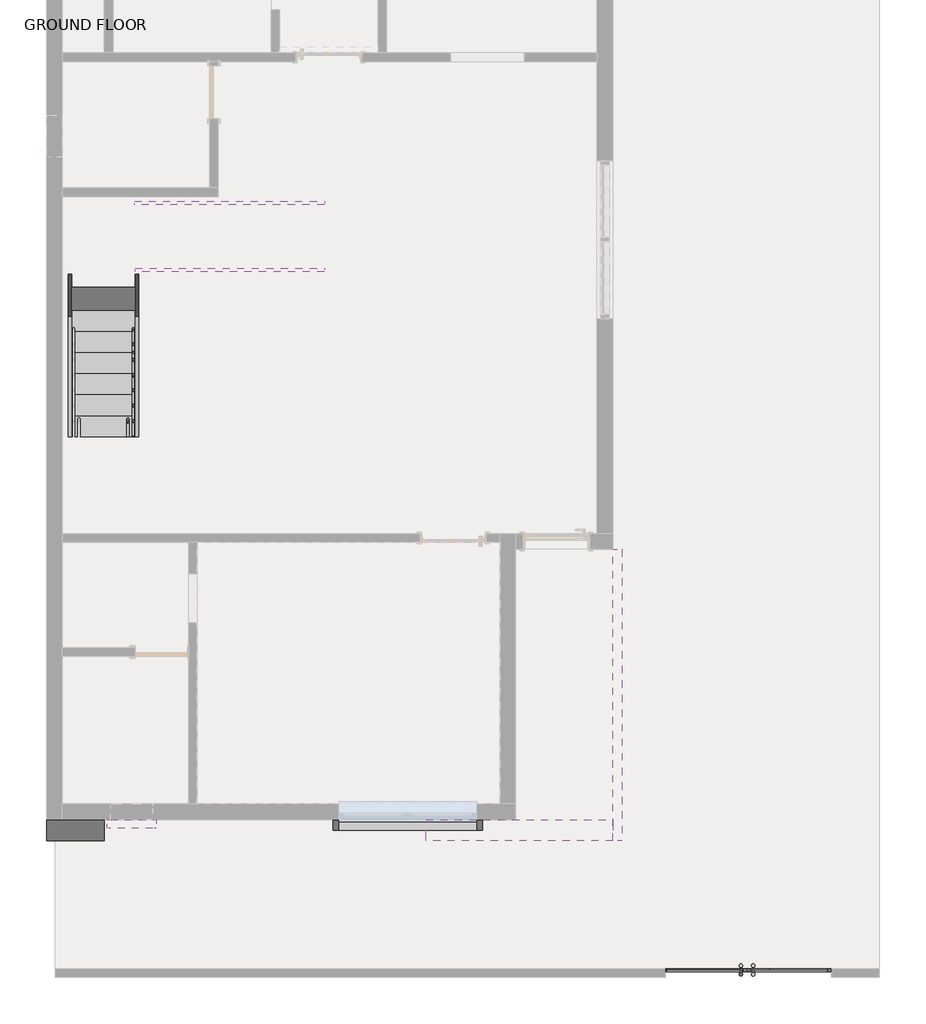
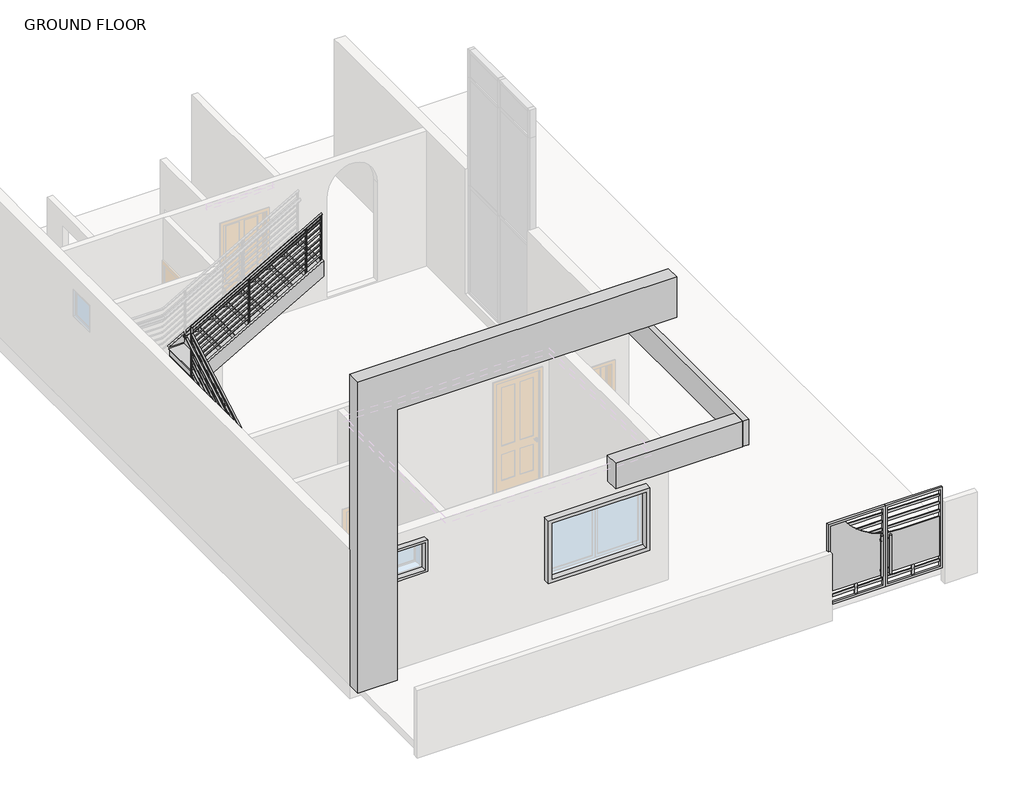
# One storey, part 3 of 3: 6 proxies, 4 members, 1 railing, 1 stair flight.
"""IFC4 building model written with IfcOpenShell, lengths in millimetres."""

from ifc_helpers import new_model, si_unit, frame, origin, place, context, project, spatial, polyline, circle_curve, ellipse_curve, outline, extrude, transform, mapped, element, save
from ifc_brep_helpers import plane_surface, cylinder_surface, advanced_brep
from components import generic_models_113f6068, generic_models_1_generic_models_1_e6ddf01a, generic_models_4_generic_models_3_1a75a499, generic_models_6_generic_models_6_7c639092, generic_models_8_generic_models_8_1b8929a2, wall_frame_wall_frame_a6ba02d1, stair_flight_5496a8fe

model = new_model("IFC4")

# Units and contexts
model_context = context("Model", 3, world=origin())
ifc_project = project(units=[si_unit("LENGTHUNIT", "METRE", prefix="MILLI")], contexts=[model_context])

# Site, building, storey
site = spatial("IfcSite", under=ifc_project)
building = spatial("IfcBuilding", under=site)
storey = spatial("IfcBuildingStorey", under=building, Name="GROUND FLOOR", Elevation=304.8)

# Proxies
placement = place(None, origin())
generic_models_shape = generic_models_113f6068(model_context)
element("IfcBuildingElementProxy", 1, Name="Generic Models", at=placement, inside=storey, context=model_context, shape_type="MappedRepresentation", body=[
    mapped(generic_models_shape, transform((2838.426752, -5931.4866303, 304.8), x_axis=(1.0, 0.0, 0.0), y_axis=(0.0, 1.0, 0.0), z_axis=(0.0, 0.0, 1.0))),
])
generic_models_1_generic_models_1_shape = generic_models_1_generic_models_1_e6ddf01a(model_context)
element("IfcBuildingElementProxy", 2, Name="Generic Models 2 : Generic Models 1", ObjectType="Generic Models 2 : Generic Models 1", at=placement, inside=storey, context=model_context, shape_type="MappedRepresentation", body=[
    mapped(generic_models_1_generic_models_1_shape, transform((0.0, 0.0, -3048.0), x_axis=(1.0, 0.0, 0.0), y_axis=(0.0, 1.0, 0.0), z_axis=(0.0, 0.0, 1.0))),
])
generic_models_4_generic_models_3_shape = generic_models_4_generic_models_3_1a75a499(model_context)
element("IfcBuildingElementProxy", 3, Name="Generic Models 4 : Generic Models 3", ObjectType="Generic Models 4 : Generic Models 3", at=placement, inside=storey, context=model_context, shape_type="MappedRepresentation", body=[
    mapped(generic_models_4_generic_models_3_shape, transform((0.0, 0.0, 0.0), x_axis=(1.0, 0.0, 0.0), y_axis=(0.0, 1.0, 0.0), z_axis=(0.0, 0.0, 1.0))),
])
generic_models_6_generic_models_6_shape = generic_models_6_generic_models_6_7c639092(model_context)
element("IfcBuildingElementProxy", 4, Name="Generic Models 6 : Generic Models 6", ObjectType="Generic Models 6 : Generic Models 6", at=placement, inside=storey, context=model_context, shape_type="MappedRepresentation", body=[
    mapped(generic_models_6_generic_models_6_shape, transform((0.0, 0.0, 0.0), x_axis=(1.0, 0.0, 0.0), y_axis=(0.0, 1.0, 0.0), z_axis=(0.0, 0.0, 1.0))),
])
generic_models_8_generic_models_8_shape = generic_models_8_generic_models_8_1b8929a2(model_context)
element("IfcBuildingElementProxy", 5, Name="Generic Models 8 : Generic Models 8", ObjectType="Generic Models 8 : Generic Models 8", at=placement, inside=storey, context=model_context, shape_type="MappedRepresentation", body=[
    mapped(generic_models_8_generic_models_8_shape, transform((0.0, 0.0, 0.0), x_axis=(1.0, 0.0, 0.0), y_axis=(0.0, 1.0, 0.0), z_axis=(0.0, 0.0, 1.0))),
])
wall_frame_wall_frame_shape = wall_frame_wall_frame_a6ba02d1(model_context)
element("IfcBuildingElementProxy", 6, Name="WALL FRAME : WALL FRAME", ObjectType="WALL FRAME : WALL FRAME", at=placement, inside=storey, context=model_context, shape_type="MappedRepresentation", body=[
    mapped(wall_frame_wall_frame_shape, transform((0.0, 0.0, 0.0), x_axis=(1.0, 0.0, 0.0), y_axis=(0.0, 1.0, 0.0), z_axis=(0.0, 0.0, 1.0))),
])

# Members
element("IfcMember", 7, ObjectType="Stringer - 2\" Width", at=placement, inside=storey, context=model_context, shape_type="SweptSolid", body=[
    extrude(outline(polyline([(1771.427543, 304.8), (1771.427543, 513.774685), (3600.227543, 1558.8032564), (4214.5715834, 1558.8032564), (2020.0658847, 304.8), (1771.427543, 304.8)])), frame((-6992.4757327, 0.0, 0.0), z_axis=(1.0, 0.0, 0.0), x_axis=(0.0, 1.0, 0.0)), (0.0, 0.0, 1.0), 50.8),
])
element("IfcMember", 8, ObjectType="Stringer - 2\" Width", at=placement, inside=storey, context=model_context, shape_type="SweptSolid", body=[
    extrude(outline(polyline([(2078.6066619, -5417.6757327), (3297.8066619, -3284.0757327), (3648.8603992, -3284.0757327), (2078.6066619, -6032.0197731), (2078.6066619, -5417.6757327)])), frame((0.0, 5124.227543, 0.0), z_axis=(0.0, 1.0, 0.0), x_axis=(0.0, 0.0, 1.0)), (0.0, 0.0, 1.0), 50.8),
])
element("IfcMember", 9, ObjectType="Stringer - 2\" Width", at=placement, inside=storey, context=model_context, shape_type="SweptSolid", body=[
    extrude(outline(polyline([(1771.427543, 304.8), (1771.427543, 513.774685), (4159.027543, 1878.1175421), (4159.027543, 1527.0638047), (2020.0658847, 304.8), (1771.427543, 304.8)])), frame((-6027.2757327, 0.0, 0.0), z_axis=(1.0, 0.0, 0.0), x_axis=(0.0, 1.0, 0.0)), (0.0, 0.0, 1.0), 50.8),
])
element("IfcMember", 10, ObjectType="Stringer - 2\" Width", at=placement, inside=storey, context=model_context, shape_type="SweptSolid", body=[
    extrude(outline(polyline([(2081.3175421, -6027.2757327), (1730.2638047, -6027.2757327), (3297.8066619, -3284.0757327), (3648.8603992, -3284.0757327), (2081.3175421, -6027.2757327)])), frame((0.0, 4159.027543, 0.0), z_axis=(0.0, 1.0, 0.0), x_axis=(0.0, 0.0, 1.0)), (0.0, 0.0, 1.0), 50.8),
])

# Railing
element("IfcRailing", 11, ObjectType="Guardrail - Pipe", at=placement, inside=storey, context=model_context, shape_type="AdvancedBrep", body=[
    advanced_brep(
    [(-6109.8257327, 1771.427543, 1371.43057), (-6147.9257327, 1771.427543, 1371.43057), (-6109.8257327, 4311.427543, 2822.8591414), (-6147.9257327, 4311.427543, 2822.8591414)],
    [
        (0, 1, ellipse_curve(frame((-6128.8757327, 1771.427543, 1371.43057), z_axis=(0.0, -1.0, 0.0), x_axis=(0.0, 0.0, -1.0)), 21.9408586, 19.05)),
        (1, 0, ellipse_curve(frame((-6128.8757327, 1771.427543, 1371.43057), z_axis=(0.0, -1.0, 0.0), x_axis=(0.0, 0.0, -1.0)), 21.9408586, 19.05)),
        (2, 3, ellipse_curve(frame((-6128.8757327, 4311.427543, 2822.8591414), z_axis=(0.0, 0.5019268181932278, 0.8649100931185983), x_axis=(0.0, -0.8649100931185982, 0.5019268181932279)), 22.0254107, 19.05)),
        (3, 2, ellipse_curve(frame((-6128.8757327, 4311.427543, 2822.8591414), z_axis=(0.0, 0.5019268181932278, 0.8649100931185983), x_axis=(0.0, -0.8649100931185982, 0.5019268181932279)), 22.0254107, 19.05)),
        (0, 2),
        (3, 1),
    ],
    [
        plane_surface(frame((-6128.8757327, 1771.427543, 1393.3714286), z_axis=(0.0, -1.0, 0.0), x_axis=(0.0, 0.0, 1.0))),
        plane_surface(frame((-6128.8757327, 4292.377543, 2833.9142857), z_axis=(0.0, 0.5019268181932278, 0.8649100931185983), x_axis=(1.0, 0.0, 0.0))),
        cylinder_surface(frame((-6128.8757327, 1780.8789898, 1376.8313967), z_axis=(0.0, -0.8682431421244483, -0.4961389383568529), x_axis=(-1.0, 0.0, 0.0)), 19.05),
    ],
    [
        (0, [[1, 2]]),
        (1, [[3, 4]]),
        (2, [[-1, 5, -4, 6]]),
        (2, [[-2, -6, -3, -5]]),
    ],
),
    advanced_brep(
    [(-6109.8257327, 4313.9375111, 2821.4025503), (-6147.9257327, 4313.9375111, 2821.4025503), (-6109.8257327, 4313.9375111, 2869.86114), (-6147.9257327, 4313.9375111, 2891.9714286)],
    [
        (0, 1, ellipse_curve(frame((-6128.8757327, 4313.9375111, 2821.4025503), z_axis=(0.0, -0.5019268181932278, -0.8649100931185983), x_axis=(0.0, 0.8649100931185985, -0.5019268181932277)), 22.0254107, 19.05)),
        (1, 0, ellipse_curve(frame((-6128.8757327, 4313.9375111, 2821.4025503), z_axis=(0.0, -0.5019268181932278, -0.8649100931185983), x_axis=(0.0, 0.8649100931185985, -0.5019268181932277)), 22.0254107, 19.05)),
        (2, 3, ellipse_curve(frame((-6128.8757327, 4313.9375111, 2880.9162843), z_axis=(0.5019268181932238, 0.0, 0.8649100931186007), x_axis=(0.8649100931186007, 0.0, -0.5019268181932236)), 22.0254107, 19.05)),
        (3, 2, ellipse_curve(frame((-6128.8757327, 4313.9375111, 2880.9162843), z_axis=(0.5019268181932238, 0.0, 0.8649100931186007), x_axis=(0.8649100931186007, 0.0, -0.5019268181932236)), 22.0254107, 19.05)),
        (0, 2),
        (3, 1),
    ],
    [
        plane_surface(frame((-6128.8757327, 4311.427543, 2822.8591414), z_axis=(0.0, -0.5019268181932278, -0.8649100931185983), x_axis=(1.0, 0.0, 0.0))),
        plane_surface(frame((-6128.8757327, 4311.427543, 2880.9162843), z_axis=(0.5019268181932238, 0.0, 0.8649100931186007), x_axis=(0.8649100931186007, 0.0, -0.5019268181932238))),
        cylinder_surface(frame((-6128.8757327, 4313.9375111, 2822.8591414), z_axis=(0.0, 0.0, -1.0), x_axis=(-1.0, 0.0, 0.0)), 19.05),
    ],
    [
        (0, [[1, 2]]),
        (1, [[3, 4]]),
        (2, [[-1, 5, -4, 6]]),
        (2, [[-2, -6, -3, -5]]),
    ],
),
    advanced_brep(
    [(-6128.8757327, 4292.377543, 2880.9162843), (-6128.8757327, 4330.477543, 2880.9162843), (-3284.0757327, 4292.377543, 4506.5162843), (-3284.0757327, 4330.477543, 4506.5162843)],
    [
        (0, 1, ellipse_curve(frame((-6128.8757327, 4311.427543, 2880.9162843), z_axis=(-0.5019268181932238, 0.0, -0.8649100931186007), x_axis=(-0.8649100931186008, 0.0, 0.5019268181932238)), 22.0254107, 19.05)),
        (1, 0, ellipse_curve(frame((-6128.8757327, 4311.427543, 2880.9162843), z_axis=(-0.5019268181932238, 0.0, -0.8649100931186007), x_axis=(-0.8649100931186008, 0.0, 0.5019268181932238)), 22.0254107, 19.05)),
        (2, 3, ellipse_curve(frame((-3284.0757327, 4311.427543, 4506.5162843), z_axis=(1.0, 0.0, 0.0), x_axis=(0.0, 0.0, -1.0)), 21.9408586, 19.05)),
        (3, 2, ellipse_curve(frame((-3284.0757327, 4311.427543, 4506.5162843), z_axis=(1.0, 0.0, 0.0), x_axis=(0.0, 0.0, -1.0)), 21.9408586, 19.05)),
        (0, 2),
        (3, 1),
    ],
    [
        plane_surface(frame((-6147.9257327, 4311.427543, 2891.9714286), z_axis=(-0.5019268181932238, 0.0, -0.8649100931186007), x_axis=(0.8649100931186007, 0.0, -0.5019268181932238))),
        plane_surface(frame((-3284.0757327, 4311.427543, 4528.4571429), z_axis=(1.0, 0.0, 0.0), x_axis=(0.0, 1.0, 0.0))),
        cylinder_surface(frame((-6138.4742859, 4311.427543, 2875.4313967), z_axis=(-0.8682431421244483, 0.0, -0.496138938356853), x_axis=(0.0, 1.0, 0.0)), 19.05),
    ],
    [
        (0, [[1, 2]]),
        (1, [[3, 4]]),
        (2, [[-1, 5, -4, 6]]),
        (2, [[-2, -6, -3, -5]]),
    ],
),
    advanced_brep(
    [(-6033.6257327, 1771.427543, 1523.83057), (-6071.7257327, 1771.427543, 1523.83057), (-6033.6257327, 4235.227543, 2931.7162843), (-6071.7257327, 4235.227543, 2931.7162843)],
    [
        (0, 1, ellipse_curve(frame((-6052.6757327, 1771.427543, 1523.83057), z_axis=(0.0, -1.0, 0.0), x_axis=(0.0, 0.0, -1.0)), 21.9408586, 19.05)),
        (1, 0, ellipse_curve(frame((-6052.6757327, 1771.427543, 1523.83057), z_axis=(0.0, -1.0, 0.0), x_axis=(0.0, 0.0, -1.0)), 21.9408586, 19.05)),
        (2, 3, ellipse_curve(frame((-6052.6757327, 4235.227543, 2931.7162843), z_axis=(0.0, 0.501926818193227, 0.8649100931185988), x_axis=(0.0, -0.8649100931185989, 0.5019268181932269)), 22.0254107, 19.05)),
        (3, 2, ellipse_curve(frame((-6052.6757327, 4235.227543, 2931.7162843), z_axis=(0.0, 0.501926818193227, 0.8649100931185988), x_axis=(0.0, -0.8649100931185989, 0.5019268181932269)), 22.0254107, 19.05)),
        (0, 2),
        (3, 1),
    ],
    [
        plane_surface(frame((-6052.6757327, 1771.427543, 1545.7714286), z_axis=(0.0, -1.0, 0.0), x_axis=(0.0, 0.0, 1.0))),
        plane_surface(frame((-6052.6757327, 4216.177543, 2942.7714286), z_axis=(0.0, 0.501926818193227, 0.8649100931185988), x_axis=(1.0, 0.0, 0.0))),
        cylinder_surface(frame((-6052.6757327, 1780.8789898, 1529.2313967), z_axis=(0.0, -0.8682431421244483, -0.4961389383568529), x_axis=(-1.0, 0.0, 0.0)), 19.05),
    ],
    [
        (0, [[1, 2]]),
        (1, [[3, 4]]),
        (2, [[-1, 5, -4, 6]]),
        (2, [[-2, -6, -3, -5]]),
    ],
),
    advanced_brep(
    [(-6033.6257327, 4237.7375111, 2930.2596932), (-6071.7257327, 4237.7375111, 2930.2596932), (-6033.6257327, 4237.7375111, 3065.8039971), (-6071.7257327, 4237.7375111, 3087.9142857)],
    [
        (0, 1, ellipse_curve(frame((-6052.6757327, 4237.7375111, 2930.2596932), z_axis=(0.0, -0.501926818193227, -0.8649100931185988), x_axis=(0.0, 0.8649100931185988, -0.5019268181932268)), 22.0254107, 19.05)),
        (1, 0, ellipse_curve(frame((-6052.6757327, 4237.7375111, 2930.2596932), z_axis=(0.0, -0.501926818193227, -0.8649100931185988), x_axis=(0.0, 0.8649100931185988, -0.5019268181932268)), 22.0254107, 19.05)),
        (2, 3, ellipse_curve(frame((-6052.6757327, 4237.7375111, 3076.8591414), z_axis=(0.5019268181932238, 0.0, 0.8649100931186007), x_axis=(0.8649100931186007, 0.0, -0.5019268181932236)), 22.0254107, 19.05)),
        (3, 2, ellipse_curve(frame((-6052.6757327, 4237.7375111, 3076.8591414), z_axis=(0.5019268181932238, 0.0, 0.8649100931186007), x_axis=(0.8649100931186007, 0.0, -0.5019268181932236)), 22.0254107, 19.05)),
        (0, 2),
        (3, 1),
    ],
    [
        plane_surface(frame((-6052.6757327, 4235.227543, 2931.7162843), z_axis=(0.0, -0.501926818193227, -0.8649100931185988), x_axis=(1.0, 0.0, 0.0))),
        plane_surface(frame((-6052.6757327, 4235.227543, 3076.8591414), z_axis=(0.5019268181932238, 0.0, 0.8649100931186007), x_axis=(0.8649100931186007, 0.0, -0.5019268181932238))),
        cylinder_surface(frame((-6052.6757327, 4237.7375111, 2931.7162843), z_axis=(0.0, 0.0, -1.0), x_axis=(-1.0, 0.0, 0.0)), 19.05),
    ],
    [
        (0, [[1, 2]]),
        (1, [[3, 4]]),
        (2, [[-1, 5, -4, 6]]),
        (2, [[-2, -6, -3, -5]]),
    ],
),
    advanced_brep(
    [(-6052.6757327, 4216.177543, 3076.8591414), (-6052.6757327, 4254.277543, 3076.8591414), (-3284.0757327, 4216.177543, 4658.9162843), (-3284.0757327, 4254.277543, 4658.9162843)],
    [
        (0, 1, ellipse_curve(frame((-6052.6757327, 4235.227543, 3076.8591414), z_axis=(-0.5019268181932238, 0.0, -0.8649100931186007), x_axis=(-0.8649100931186008, 0.0, 0.5019268181932238)), 22.0254107, 19.05)),
        (1, 0, ellipse_curve(frame((-6052.6757327, 4235.227543, 3076.8591414), z_axis=(-0.5019268181932238, 0.0, -0.8649100931186007), x_axis=(-0.8649100931186008, 0.0, 0.5019268181932238)), 22.0254107, 19.05)),
        (2, 3, ellipse_curve(frame((-3284.0757327, 4235.227543, 4658.9162843), z_axis=(1.0, 0.0, 0.0), x_axis=(0.0, 0.0, -1.0)), 21.9408586, 19.05)),
        (3, 2, ellipse_curve(frame((-3284.0757327, 4235.227543, 4658.9162843), z_axis=(1.0, 0.0, 0.0), x_axis=(0.0, 0.0, -1.0)), 21.9408586, 19.05)),
        (0, 2),
        (3, 1),
    ],
    [
        plane_surface(frame((-6071.7257327, 4235.227543, 3087.9142857), z_axis=(-0.5019268181932238, 0.0, -0.8649100931186007), x_axis=(0.8649100931186007, 0.0, -0.5019268181932238))),
        plane_surface(frame((-3284.0757327, 4235.227543, 4680.8571429), z_axis=(1.0, 0.0, 0.0), x_axis=(0.0, 1.0, 0.0))),
        cylinder_surface(frame((-6062.2742859, 4235.227543, 3071.3742539), z_axis=(-0.8682431421244483, 0.0, -0.496138938356853), x_axis=(0.0, 1.0, 0.0)), 19.05),
    ],
    [
        (0, [[1, 2]]),
        (1, [[3, 4]]),
        (2, [[-1, 5, -4, 6]]),
        (2, [[-2, -6, -3, -5]]),
    ],
),
    advanced_brep(
    [(-6065.3757327, 1771.427543, 1378.7441895), (-6039.9757327, 1771.427543, 1378.7441895), (-6065.3757327, 4222.527543, 2779.3727609), (-6039.9757327, 4222.527543, 2779.3727609)],
    [
        (0, 1, ellipse_curve(frame((-6052.6757327, 1771.427543, 1378.7441895), z_axis=(0.0, -1.0, 0.0), x_axis=(0.0, 0.0, -1.0)), 14.6272391, 12.7)),
        (1, 0, ellipse_curve(frame((-6052.6757327, 1771.427543, 1378.7441895), z_axis=(0.0, -1.0, 0.0), x_axis=(0.0, 0.0, -1.0)), 14.6272391, 12.7)),
        (2, 3, ellipse_curve(frame((-6052.6757327, 4222.527543, 2779.3727609), z_axis=(0.0, 1.0, 0.0), x_axis=(0.0, 0.0, -1.0)), 14.6272391, 12.7)),
        (3, 2, ellipse_curve(frame((-6052.6757327, 4222.527543, 2779.3727609), z_axis=(0.0, 1.0, 0.0), x_axis=(0.0, 0.0, -1.0)), 14.6272391, 12.7)),
        (0, 2),
        (3, 1),
    ],
    [
        plane_surface(frame((-6052.6757327, 1771.427543, 1393.3714286), z_axis=(0.0, -1.0, 0.0), x_axis=(0.0, 0.0, 1.0))),
        plane_surface(frame((-6052.6757327, 4222.527543, 2794.0), z_axis=(0.0, 1.0, 0.0), x_axis=(0.0, 0.0, 1.0))),
        cylinder_surface(frame((-6052.6757327, 1777.7285075, 1382.3447407), z_axis=(0.0, -0.8682431421244483, -0.4961389383568529), x_axis=(1.0, 0.0, 0.0)), 12.7),
    ],
    [
        (0, [[1, 2]]),
        (1, [[3, 4]]),
        (2, [[-1, 5, -4, 6]]),
        (2, [[-2, -6, -3, -5]]),
    ],
),
    advanced_brep(
    [(-6065.3757327, 4247.927543, 2924.5156181), (-6065.3757327, 4222.527543, 2924.5156181), (-3284.0757327, 4247.927543, 4513.8299038), (-3284.0757327, 4222.527543, 4513.8299038)],
    [
        (0, 1, ellipse_curve(frame((-6065.3757327, 4235.227543, 2924.5156181), z_axis=(-1.0, 0.0, 0.0), x_axis=(0.0, 0.0, -1.0)), 14.6272391, 12.7)),
        (1, 0, ellipse_curve(frame((-6065.3757327, 4235.227543, 2924.5156181), z_axis=(-1.0, 0.0, 0.0), x_axis=(0.0, 0.0, -1.0)), 14.6272391, 12.7)),
        (2, 3, ellipse_curve(frame((-3284.0757327, 4235.227543, 4513.8299038), z_axis=(1.0, 0.0, 0.0), x_axis=(0.0, 0.0, -1.0)), 14.6272391, 12.7)),
        (3, 2, ellipse_curve(frame((-3284.0757327, 4235.227543, 4513.8299038), z_axis=(1.0, 0.0, 0.0), x_axis=(0.0, 0.0, -1.0)), 14.6272391, 12.7)),
        (0, 2),
        (3, 1),
    ],
    [
        plane_surface(frame((-6065.3757327, 4235.227543, 2939.1428571), z_axis=(-1.0, 0.0, 0.0), x_axis=(0.0, 1.0, 0.0))),
        plane_surface(frame((-3284.0757327, 4235.227543, 4528.4571429), z_axis=(1.0, 0.0, 0.0), x_axis=(0.0, 1.0, 0.0))),
        cylinder_surface(frame((-6059.0747682, 4235.227543, 2928.1161692), z_axis=(-0.8682431421244483, 0.0, -0.496138938356853), x_axis=(0.0, -1.0, 0.0)), 12.7),
    ],
    [
        (0, [[1, 2]]),
        (1, [[3, 4]]),
        (2, [[-1, 5, -4, 6]]),
        (2, [[-2, -6, -3, -5]]),
    ],
),
    advanced_brep(
    [(-6065.3757327, 1771.427543, 1251.7441895), (-6039.9757327, 1771.427543, 1251.7441895), (-6065.3757327, 4222.527543, 2652.3727609), (-6039.9757327, 4222.527543, 2652.3727609)],
    [
        (0, 1, ellipse_curve(frame((-6052.6757327, 1771.427543, 1251.7441895), z_axis=(0.0, -1.0, 0.0), x_axis=(0.0, 0.0, -1.0)), 14.6272391, 12.7)),
        (1, 0, ellipse_curve(frame((-6052.6757327, 1771.427543, 1251.7441895), z_axis=(0.0, -1.0, 0.0), x_axis=(0.0, 0.0, -1.0)), 14.6272391, 12.7)),
        (2, 3, ellipse_curve(frame((-6052.6757327, 4222.527543, 2652.3727609), z_axis=(0.0, 1.0, 0.0), x_axis=(0.0, 0.0, -1.0)), 14.6272391, 12.7)),
        (3, 2, ellipse_curve(frame((-6052.6757327, 4222.527543, 2652.3727609), z_axis=(0.0, 1.0, 0.0), x_axis=(0.0, 0.0, -1.0)), 14.6272391, 12.7)),
        (0, 2),
        (3, 1),
    ],
    [
        plane_surface(frame((-6052.6757327, 1771.427543, 1266.3714286), z_axis=(0.0, -1.0, 0.0), x_axis=(0.0, 0.0, 1.0))),
        plane_surface(frame((-6052.6757327, 4222.527543, 2667.0), z_axis=(0.0, 1.0, 0.0), x_axis=(0.0, 0.0, 1.0))),
        cylinder_surface(frame((-6052.6757327, 1777.7285075, 1255.3447407), z_axis=(0.0, -0.8682431421244483, -0.4961389383568529), x_axis=(1.0, 0.0, 0.0)), 12.7),
    ],
    [
        (0, [[1, 2]]),
        (1, [[3, 4]]),
        (2, [[-1, 5, -4, 6]]),
        (2, [[-2, -6, -3, -5]]),
    ],
),
    advanced_brep(
    [(-6065.3757327, 4247.927543, 2797.5156181), (-6065.3757327, 4222.527543, 2797.5156181), (-3284.0757327, 4247.927543, 4386.8299038), (-3284.0757327, 4222.527543, 4386.8299038)],
    [
        (0, 1, ellipse_curve(frame((-6065.3757327, 4235.227543, 2797.5156181), z_axis=(-1.0, 0.0, 0.0), x_axis=(0.0, 0.0, -1.0)), 14.6272391, 12.7)),
        (1, 0, ellipse_curve(frame((-6065.3757327, 4235.227543, 2797.5156181), z_axis=(-1.0, 0.0, 0.0), x_axis=(0.0, 0.0, -1.0)), 14.6272391, 12.7)),
        (2, 3, ellipse_curve(frame((-3284.0757327, 4235.227543, 4386.8299038), z_axis=(1.0, 0.0, 0.0), x_axis=(0.0, 0.0, -1.0)), 14.6272391, 12.7)),
        (3, 2, ellipse_curve(frame((-3284.0757327, 4235.227543, 4386.8299038), z_axis=(1.0, 0.0, 0.0), x_axis=(0.0, 0.0, -1.0)), 14.6272391, 12.7)),
        (0, 2),
        (3, 1),
    ],
    [
        plane_surface(frame((-6065.3757327, 4235.227543, 2812.1428571), z_axis=(-1.0, 0.0, 0.0), x_axis=(0.0, 1.0, 0.0))),
        plane_surface(frame((-3284.0757327, 4235.227543, 4401.4571429), z_axis=(1.0, 0.0, 0.0), x_axis=(0.0, 1.0, 0.0))),
        cylinder_surface(frame((-6059.0747682, 4235.227543, 2801.1161692), z_axis=(-0.8682431421244483, 0.0, -0.496138938356853), x_axis=(0.0, -1.0, 0.0)), 12.7),
    ],
    [
        (0, [[1, 2]]),
        (1, [[3, 4]]),
        (2, [[-1, 5, -4, 6]]),
        (2, [[-2, -6, -3, -5]]),
    ],
),
    advanced_brep(
    [(-6065.3757327, 1771.427543, 1124.7441895), (-6039.9757327, 1771.427543, 1124.7441895), (-6065.3757327, 4222.527543, 2525.3727609), (-6039.9757327, 4222.527543, 2525.3727609)],
    [
        (0, 1, ellipse_curve(frame((-6052.6757327, 1771.427543, 1124.7441895), z_axis=(0.0, -1.0, 0.0), x_axis=(0.0, 0.0, -1.0)), 14.6272391, 12.7)),
        (1, 0, ellipse_curve(frame((-6052.6757327, 1771.427543, 1124.7441895), z_axis=(0.0, -1.0, 0.0), x_axis=(0.0, 0.0, -1.0)), 14.6272391, 12.7)),
        (2, 3, ellipse_curve(frame((-6052.6757327, 4222.527543, 2525.3727609), z_axis=(0.0, 1.0, 0.0), x_axis=(0.0, 0.0, -1.0)), 14.6272391, 12.7)),
        (3, 2, ellipse_curve(frame((-6052.6757327, 4222.527543, 2525.3727609), z_axis=(0.0, 1.0, 0.0), x_axis=(0.0, 0.0, -1.0)), 14.6272391, 12.7)),
        (0, 2),
        (3, 1),
    ],
    [
        plane_surface(frame((-6052.6757327, 1771.427543, 1139.3714286), z_axis=(0.0, -1.0, 0.0), x_axis=(0.0, 0.0, 1.0))),
        plane_surface(frame((-6052.6757327, 4222.527543, 2540.0), z_axis=(0.0, 1.0, 0.0), x_axis=(0.0, 0.0, 1.0))),
        cylinder_surface(frame((-6052.6757327, 1777.7285075, 1128.3447407), z_axis=(0.0, -0.8682431421244483, -0.4961389383568529), x_axis=(1.0, 0.0, 0.0)), 12.7),
    ],
    [
        (0, [[1, 2]]),
        (1, [[3, 4]]),
        (2, [[-1, 5, -4, 6]]),
        (2, [[-2, -6, -3, -5]]),
    ],
),
    advanced_brep(
    [(-6065.3757327, 4247.927543, 2670.5156181), (-6065.3757327, 4222.527543, 2670.5156181), (-3284.0757327, 4247.927543, 4259.8299038), (-3284.0757327, 4222.527543, 4259.8299038)],
    [
        (0, 1, ellipse_curve(frame((-6065.3757327, 4235.227543, 2670.5156181), z_axis=(-1.0, 0.0, 0.0), x_axis=(0.0, 0.0, -1.0)), 14.6272391, 12.7)),
        (1, 0, ellipse_curve(frame((-6065.3757327, 4235.227543, 2670.5156181), z_axis=(-1.0, 0.0, 0.0), x_axis=(0.0, 0.0, -1.0)), 14.6272391, 12.7)),
        (2, 3, ellipse_curve(frame((-3284.0757327, 4235.227543, 4259.8299038), z_axis=(1.0, 0.0, 0.0), x_axis=(0.0, 0.0, -1.0)), 14.6272391, 12.7)),
        (3, 2, ellipse_curve(frame((-3284.0757327, 4235.227543, 4259.8299038), z_axis=(1.0, 0.0, 0.0), x_axis=(0.0, 0.0, -1.0)), 14.6272391, 12.7)),
        (0, 2),
        (3, 1),
    ],
    [
        plane_surface(frame((-6065.3757327, 4235.227543, 2685.1428571), z_axis=(-1.0, 0.0, 0.0), x_axis=(0.0, 1.0, 0.0))),
        plane_surface(frame((-3284.0757327, 4235.227543, 4274.4571429), z_axis=(1.0, 0.0, 0.0), x_axis=(0.0, 1.0, 0.0))),
        cylinder_surface(frame((-6059.0747682, 4235.227543, 2674.1161692), z_axis=(-0.8682431421244483, 0.0, -0.496138938356853), x_axis=(0.0, -1.0, 0.0)), 12.7),
    ],
    [
        (0, [[1, 2]]),
        (1, [[3, 4]]),
        (2, [[-1, 5, -4, 6]]),
        (2, [[-2, -6, -3, -5]]),
    ],
),
    advanced_brep(
    [(-6065.3757327, 1771.427543, 997.7441895), (-6039.9757327, 1771.427543, 997.7441895), (-6065.3757327, 4222.527543, 2398.3727609), (-6039.9757327, 4222.527543, 2398.3727609)],
    [
        (0, 1, ellipse_curve(frame((-6052.6757327, 1771.427543, 997.7441895), z_axis=(0.0, -1.0, 0.0), x_axis=(0.0, 0.0, -1.0)), 14.6272391, 12.7)),
        (1, 0, ellipse_curve(frame((-6052.6757327, 1771.427543, 997.7441895), z_axis=(0.0, -1.0, 0.0), x_axis=(0.0, 0.0, -1.0)), 14.6272391, 12.7)),
        (2, 3, ellipse_curve(frame((-6052.6757327, 4222.527543, 2398.3727609), z_axis=(0.0, 1.0, 0.0), x_axis=(0.0, 0.0, -1.0)), 14.6272391, 12.7)),
        (3, 2, ellipse_curve(frame((-6052.6757327, 4222.527543, 2398.3727609), z_axis=(0.0, 1.0, 0.0), x_axis=(0.0, 0.0, -1.0)), 14.6272391, 12.7)),
        (0, 2),
        (3, 1),
    ],
    [
        plane_surface(frame((-6052.6757327, 1771.427543, 1012.3714286), z_axis=(0.0, -1.0, 0.0), x_axis=(0.0, 0.0, 1.0))),
        plane_surface(frame((-6052.6757327, 4222.527543, 2413.0), z_axis=(0.0, 1.0, 0.0), x_axis=(0.0, 0.0, 1.0))),
        cylinder_surface(frame((-6052.6757327, 1777.7285075, 1001.3447407), z_axis=(0.0, -0.8682431421244483, -0.4961389383568529), x_axis=(1.0, 0.0, 0.0)), 12.7),
    ],
    [
        (0, [[1, 2]]),
        (1, [[3, 4]]),
        (2, [[-1, 5, -4, 6]]),
        (2, [[-2, -6, -3, -5]]),
    ],
),
    advanced_brep(
    [(-6065.3757327, 4247.927543, 2543.5156181), (-6065.3757327, 4222.527543, 2543.5156181), (-3284.0757327, 4247.927543, 4132.8299038), (-3284.0757327, 4222.527543, 4132.8299038)],
    [
        (0, 1, ellipse_curve(frame((-6065.3757327, 4235.227543, 2543.5156181), z_axis=(-1.0, 0.0, 0.0), x_axis=(0.0, 0.0, -1.0)), 14.6272391, 12.7)),
        (1, 0, ellipse_curve(frame((-6065.3757327, 4235.227543, 2543.5156181), z_axis=(-1.0, 0.0, 0.0), x_axis=(0.0, 0.0, -1.0)), 14.6272391, 12.7)),
        (2, 3, ellipse_curve(frame((-3284.0757327, 4235.227543, 4132.8299038), z_axis=(1.0, 0.0, 0.0), x_axis=(0.0, 0.0, -1.0)), 14.6272391, 12.7)),
        (3, 2, ellipse_curve(frame((-3284.0757327, 4235.227543, 4132.8299038), z_axis=(1.0, 0.0, 0.0), x_axis=(0.0, 0.0, -1.0)), 14.6272391, 12.7)),
        (0, 2),
        (3, 1),
    ],
    [
        plane_surface(frame((-6065.3757327, 4235.227543, 2558.1428571), z_axis=(-1.0, 0.0, 0.0), x_axis=(0.0, 1.0, 0.0))),
        plane_surface(frame((-3284.0757327, 4235.227543, 4147.4571429), z_axis=(1.0, 0.0, 0.0), x_axis=(0.0, 1.0, 0.0))),
        cylinder_surface(frame((-6059.0747682, 4235.227543, 2547.1161692), z_axis=(-0.8682431421244483, 0.0, -0.496138938356853), x_axis=(0.0, -1.0, 0.0)), 12.7),
    ],
    [
        (0, [[1, 2]]),
        (1, [[3, 4]]),
        (2, [[-1, 5, -4, 6]]),
        (2, [[-2, -6, -3, -5]]),
    ],
),
    advanced_brep(
    [(-6065.3757327, 1771.427543, 870.7441895), (-6039.9757327, 1771.427543, 870.7441895), (-6065.3757327, 4222.527543, 2271.3727609), (-6039.9757327, 4222.527543, 2271.3727609)],
    [
        (0, 1, ellipse_curve(frame((-6052.6757327, 1771.427543, 870.7441895), z_axis=(0.0, -1.0, 0.0), x_axis=(0.0, 0.0, -1.0)), 14.6272391, 12.7)),
        (1, 0, ellipse_curve(frame((-6052.6757327, 1771.427543, 870.7441895), z_axis=(0.0, -1.0, 0.0), x_axis=(0.0, 0.0, -1.0)), 14.6272391, 12.7)),
        (2, 3, ellipse_curve(frame((-6052.6757327, 4222.527543, 2271.3727609), z_axis=(0.0, 1.0, 0.0), x_axis=(0.0, 0.0, -1.0)), 14.6272391, 12.7)),
        (3, 2, ellipse_curve(frame((-6052.6757327, 4222.527543, 2271.3727609), z_axis=(0.0, 1.0, 0.0), x_axis=(0.0, 0.0, -1.0)), 14.6272391, 12.7)),
        (0, 2),
        (3, 1),
    ],
    [
        plane_surface(frame((-6052.6757327, 1771.427543, 885.3714286), z_axis=(0.0, -1.0, 0.0), x_axis=(0.0, 0.0, 1.0))),
        plane_surface(frame((-6052.6757327, 4222.527543, 2286.0), z_axis=(0.0, 1.0, 0.0), x_axis=(0.0, 0.0, 1.0))),
        cylinder_surface(frame((-6052.6757327, 1777.7285075, 874.3447407), z_axis=(0.0, -0.8682431421244483, -0.4961389383568529), x_axis=(1.0, 0.0, 0.0)), 12.7),
    ],
    [
        (0, [[1, 2]]),
        (1, [[3, 4]]),
        (2, [[-1, 5, -4, 6]]),
        (2, [[-2, -6, -3, -5]]),
    ],
),
    advanced_brep(
    [(-6065.3757327, 4247.927543, 2416.5156181), (-6065.3757327, 4222.527543, 2416.5156181), (-3284.0757327, 4247.927543, 4005.8299038), (-3284.0757327, 4222.527543, 4005.8299038)],
    [
        (0, 1, ellipse_curve(frame((-6065.3757327, 4235.227543, 2416.5156181), z_axis=(-1.0, 0.0, 0.0), x_axis=(0.0, 0.0, -1.0)), 14.6272391, 12.7)),
        (1, 0, ellipse_curve(frame((-6065.3757327, 4235.227543, 2416.5156181), z_axis=(-1.0, 0.0, 0.0), x_axis=(0.0, 0.0, -1.0)), 14.6272391, 12.7)),
        (2, 3, ellipse_curve(frame((-3284.0757327, 4235.227543, 4005.8299038), z_axis=(1.0, 0.0, 0.0), x_axis=(0.0, 0.0, -1.0)), 14.6272391, 12.7)),
        (3, 2, ellipse_curve(frame((-3284.0757327, 4235.227543, 4005.8299038), z_axis=(1.0, 0.0, 0.0), x_axis=(0.0, 0.0, -1.0)), 14.6272391, 12.7)),
        (0, 2),
        (3, 1),
    ],
    [
        plane_surface(frame((-6065.3757327, 4235.227543, 2431.1428571), z_axis=(-1.0, 0.0, 0.0), x_axis=(0.0, 1.0, 0.0))),
        plane_surface(frame((-3284.0757327, 4235.227543, 4020.4571429), z_axis=(1.0, 0.0, 0.0), x_axis=(0.0, 1.0, 0.0))),
        cylinder_surface(frame((-6059.0747682, 4235.227543, 2420.1161692), z_axis=(-0.8682431421244483, 0.0, -0.496138938356853), x_axis=(0.0, -1.0, 0.0)), 12.7),
    ],
    [
        (0, [[1, 2]]),
        (1, [[3, 4]]),
        (2, [[-1, 5, -4, 6]]),
        (2, [[-2, -6, -3, -5]]),
    ],
),
    advanced_brep(
    [(-6065.3757327, 1771.427543, 743.7441895), (-6039.9757327, 1771.427543, 743.7441895), (-6065.3757327, 4222.527543, 2144.3727609), (-6039.9757327, 4222.527543, 2144.3727609)],
    [
        (0, 1, ellipse_curve(frame((-6052.6757327, 1771.427543, 743.7441895), z_axis=(0.0, -1.0, 0.0), x_axis=(0.0, 0.0, -1.0)), 14.6272391, 12.7)),
        (1, 0, ellipse_curve(frame((-6052.6757327, 1771.427543, 743.7441895), z_axis=(0.0, -1.0, 0.0), x_axis=(0.0, 0.0, -1.0)), 14.6272391, 12.7)),
        (2, 3, ellipse_curve(frame((-6052.6757327, 4222.527543, 2144.3727609), z_axis=(0.0, 1.0, 0.0), x_axis=(0.0, 0.0, -1.0)), 14.6272391, 12.7)),
        (3, 2, ellipse_curve(frame((-6052.6757327, 4222.527543, 2144.3727609), z_axis=(0.0, 1.0, 0.0), x_axis=(0.0, 0.0, -1.0)), 14.6272391, 12.7)),
        (0, 2),
        (3, 1),
    ],
    [
        plane_surface(frame((-6052.6757327, 1771.427543, 758.3714286), z_axis=(0.0, -1.0, 0.0), x_axis=(0.0, 0.0, 1.0))),
        plane_surface(frame((-6052.6757327, 4222.527543, 2159.0), z_axis=(0.0, 1.0, 0.0), x_axis=(0.0, 0.0, 1.0))),
        cylinder_surface(frame((-6052.6757327, 1777.7285075, 747.3447407), z_axis=(0.0, -0.8682431421244483, -0.4961389383568529), x_axis=(1.0, 0.0, 0.0)), 12.7),
    ],
    [
        (0, [[1, 2]]),
        (1, [[3, 4]]),
        (2, [[-1, 5, -4, 6]]),
        (2, [[-2, -6, -3, -5]]),
    ],
),
    advanced_brep(
    [(-6065.3757327, 4247.927543, 2289.5156181), (-6065.3757327, 4222.527543, 2289.5156181), (-3284.0757327, 4247.927543, 3878.8299038), (-3284.0757327, 4222.527543, 3878.8299038)],
    [
        (0, 1, ellipse_curve(frame((-6065.3757327, 4235.227543, 2289.5156181), z_axis=(-1.0, 0.0, 0.0), x_axis=(0.0, 0.0, -1.0)), 14.6272391, 12.7)),
        (1, 0, ellipse_curve(frame((-6065.3757327, 4235.227543, 2289.5156181), z_axis=(-1.0, 0.0, 0.0), x_axis=(0.0, 0.0, -1.0)), 14.6272391, 12.7)),
        (2, 3, ellipse_curve(frame((-3284.0757327, 4235.227543, 3878.8299038), z_axis=(1.0, 0.0, 0.0), x_axis=(0.0, 0.0, -1.0)), 14.6272391, 12.7)),
        (3, 2, ellipse_curve(frame((-3284.0757327, 4235.227543, 3878.8299038), z_axis=(1.0, 0.0, 0.0), x_axis=(0.0, 0.0, -1.0)), 14.6272391, 12.7)),
        (0, 2),
        (3, 1),
    ],
    [
        plane_surface(frame((-6065.3757327, 4235.227543, 2304.1428571), z_axis=(-1.0, 0.0, 0.0), x_axis=(0.0, 1.0, 0.0))),
        plane_surface(frame((-3284.0757327, 4235.227543, 3893.4571429), z_axis=(1.0, 0.0, 0.0), x_axis=(0.0, 1.0, 0.0))),
        cylinder_surface(frame((-6059.0747682, 4235.227543, 2293.1161692), z_axis=(-0.8682431421244483, 0.0, -0.496138938356853), x_axis=(0.0, -1.0, 0.0)), 12.7),
    ],
    [
        (0, [[1, 2]]),
        (1, [[3, 4]]),
        (2, [[-1, 5, -4, 6]]),
        (2, [[-2, -6, -3, -5]]),
    ],
),
    advanced_brep(
    [(-6065.3757327, 1771.427543, 616.7441895), (-6039.9757327, 1771.427543, 616.7441895), (-6065.3757327, 4222.527543, 2017.3727609), (-6039.9757327, 4222.527543, 2017.3727609)],
    [
        (0, 1, ellipse_curve(frame((-6052.6757327, 1771.427543, 616.7441895), z_axis=(0.0, -1.0, 0.0), x_axis=(0.0, 0.0, -1.0)), 14.6272391, 12.7)),
        (1, 0, ellipse_curve(frame((-6052.6757327, 1771.427543, 616.7441895), z_axis=(0.0, -1.0, 0.0), x_axis=(0.0, 0.0, -1.0)), 14.6272391, 12.7)),
        (2, 3, ellipse_curve(frame((-6052.6757327, 4222.527543, 2017.3727609), z_axis=(0.0, 1.0, 0.0), x_axis=(0.0, 0.0, -1.0)), 14.6272391, 12.7)),
        (3, 2, ellipse_curve(frame((-6052.6757327, 4222.527543, 2017.3727609), z_axis=(0.0, 1.0, 0.0), x_axis=(0.0, 0.0, -1.0)), 14.6272391, 12.7)),
        (0, 2),
        (3, 1),
    ],
    [
        plane_surface(frame((-6052.6757327, 1771.427543, 631.3714286), z_axis=(0.0, -1.0, 0.0), x_axis=(0.0, 0.0, 1.0))),
        plane_surface(frame((-6052.6757327, 4222.527543, 2032.0), z_axis=(0.0, 1.0, 0.0), x_axis=(0.0, 0.0, 1.0))),
        cylinder_surface(frame((-6052.6757327, 1777.7285075, 620.3447407), z_axis=(0.0, -0.8682431421244483, -0.4961389383568529), x_axis=(1.0, 0.0, 0.0)), 12.7),
    ],
    [
        (0, [[1, 2]]),
        (1, [[3, 4]]),
        (2, [[-1, 5, -4, 6]]),
        (2, [[-2, -6, -3, -5]]),
    ],
),
    advanced_brep(
    [(-6065.3757327, 4247.927543, 2162.5156181), (-6065.3757327, 4222.527543, 2162.5156181), (-3284.0757327, 4247.927543, 3751.8299038), (-3284.0757327, 4222.527543, 3751.8299038)],
    [
        (0, 1, ellipse_curve(frame((-6065.3757327, 4235.227543, 2162.5156181), z_axis=(-1.0, 0.0, 0.0), x_axis=(0.0, 0.0, -1.0)), 14.6272391, 12.7)),
        (1, 0, ellipse_curve(frame((-6065.3757327, 4235.227543, 2162.5156181), z_axis=(-1.0, 0.0, 0.0), x_axis=(0.0, 0.0, -1.0)), 14.6272391, 12.7)),
        (2, 3, ellipse_curve(frame((-3284.0757327, 4235.227543, 3751.8299038), z_axis=(1.0, 0.0, 0.0), x_axis=(0.0, 0.0, -1.0)), 14.6272391, 12.7)),
        (3, 2, ellipse_curve(frame((-3284.0757327, 4235.227543, 3751.8299038), z_axis=(1.0, 0.0, 0.0), x_axis=(0.0, 0.0, -1.0)), 14.6272391, 12.7)),
        (0, 2),
        (3, 1),
    ],
    [
        plane_surface(frame((-6065.3757327, 4235.227543, 2177.1428571), z_axis=(-1.0, 0.0, 0.0), x_axis=(0.0, 1.0, 0.0))),
        plane_surface(frame((-3284.0757327, 4235.227543, 3766.4571429), z_axis=(1.0, 0.0, 0.0), x_axis=(0.0, 1.0, 0.0))),
        cylinder_surface(frame((-6059.0747682, 4235.227543, 2166.1161692), z_axis=(-0.8682431421244483, 0.0, -0.496138938356853), x_axis=(0.0, -1.0, 0.0)), 12.7),
    ],
    [
        (0, [[1, 2]]),
        (1, [[3, 4]]),
        (2, [[-1, 5, -4, 6]]),
        (2, [[-2, -6, -3, -5]]),
    ],
),
    advanced_brep(
    [(-3614.2757327, 4222.527543, 4448.2897114), (-3614.2757327, 4222.527543, 3265.7142857), (-3614.2757327, 4247.927543, 3265.7142857), (-3614.2757327, 4247.927543, 4448.2897114)],
    [
        (0, 1),
        (1, 2, circle_curve(frame((-3614.2757327, 4235.227543, 3265.7142857), z_axis=(0.0, 0.0, 1.0), x_axis=(0.0, 1.0, 0.0)), 12.7)),
        (2, 3),
        (3, 0, ellipse_curve(frame((-3614.2757327, 4235.227543, 4448.2897114), z_axis=(0.4961389383568517, 0.0, -0.8682431421244491), x_axis=(0.8682431421244492, 0.0, 0.49613893835685136)), 14.6272391, 12.7)),
        (0, 3, ellipse_curve(frame((-3614.2757327, 4235.227543, 4448.2897114), z_axis=(0.4961389383568517, 0.0, -0.8682431421244491), x_axis=(0.8682431421244492, 0.0, 0.49613893835685136)), 14.6272391, 12.7)),
        (2, 1, circle_curve(frame((-3614.2757327, 4235.227543, 3265.7142857), z_axis=(0.0, 0.0, 1.0), x_axis=(0.0, 1.0, 0.0)), 12.7)),
    ],
    [
        cylinder_surface(frame((-3614.2757327, 4235.227543, 3037.1142857), z_axis=(0.0, 0.0, 1.0), x_axis=(0.0, 1.0, 0.0)), 12.7),
        plane_surface(frame((-3588.8757327, 4260.627543, 4462.8039971), z_axis=(-0.4961389383568517, 0.0, 0.8682431421244491), x_axis=(0.0, -1.0, 0.0))),
        plane_surface(frame((-3639.6757327, 4260.627543, 3265.7142857), z_axis=(0.0, 0.0, -1.0), x_axis=(0.0, -1.0, 0.0))),
    ],
    [
        (0, [[1, 2, 3, 4]]),
        (0, [[-1, 5, -3, 6]]),
        (1, [[-4, -5]]),
        (2, [[-2, -6]]),
    ],
),
    advanced_brep(
    [(-4833.4757327, 4222.527543, 3751.6039971), (-4833.4757327, 4222.527543, 2569.0285714), (-4833.4757327, 4247.927543, 2569.0285714), (-4833.4757327, 4247.927543, 3751.6039971)],
    [
        (0, 1),
        (1, 2, circle_curve(frame((-4833.4757327, 4235.227543, 2569.0285714), z_axis=(0.0, 0.0, 1.0), x_axis=(0.0, 1.0, 0.0)), 12.7)),
        (2, 3),
        (3, 0, ellipse_curve(frame((-4833.4757327, 4235.227543, 3751.6039971), z_axis=(0.4961389383568517, 0.0, -0.8682431421244491), x_axis=(0.8682431421244492, 0.0, 0.49613893835685136)), 14.6272391, 12.7)),
        (0, 3, ellipse_curve(frame((-4833.4757327, 4235.227543, 3751.6039971), z_axis=(0.4961389383568517, 0.0, -0.8682431421244491), x_axis=(0.8682431421244492, 0.0, 0.49613893835685136)), 14.6272391, 12.7)),
        (2, 1, circle_curve(frame((-4833.4757327, 4235.227543, 2569.0285714), z_axis=(0.0, 0.0, 1.0), x_axis=(0.0, 1.0, 0.0)), 12.7)),
    ],
    [
        cylinder_surface(frame((-4833.4757327, 4235.227543, 2340.4285714), z_axis=(0.0, 0.0, 1.0), x_axis=(0.0, 1.0, 0.0)), 12.7),
        plane_surface(frame((-4808.0757327, 4260.627543, 3766.1182828), z_axis=(-0.4961389383568517, 0.0, 0.8682431421244491), x_axis=(0.0, -1.0, 0.0))),
        plane_surface(frame((-4858.8757327, 4260.627543, 2569.0285714), z_axis=(0.0, 0.0, -1.0), x_axis=(0.0, -1.0, 0.0))),
    ],
    [
        (0, [[1, 2, 3, 4]]),
        (0, [[-1, 5, -3, 6]]),
        (1, [[-4, -5]]),
        (2, [[-2, -6]]),
    ],
),
    advanced_brep(
    [(-6039.9757327, 4209.827543, 2895.26114), (-6039.9757327, 4209.827543, 1872.3428571), (-6065.3757327, 4209.827543, 1872.3428571), (-6065.3757327, 4209.827543, 2895.26114)],
    [
        (0, 1),
        (1, 2, circle_curve(frame((-6052.6757327, 4209.827543, 1872.3428571), z_axis=(0.0, 0.0, 1.0), x_axis=(-1.0, 0.0, 0.0)), 12.7)),
        (2, 3),
        (3, 0, ellipse_curve(frame((-6052.6757327, 4209.827543, 2895.26114), z_axis=(0.0, 0.4961389383568517, -0.8682431421244491), x_axis=(0.0, 0.8682431421244492, 0.49613893835685136)), 14.6272391, 12.7)),
        (0, 3, ellipse_curve(frame((-6052.6757327, 4209.827543, 2895.26114), z_axis=(0.0, 0.4961389383568517, -0.8682431421244491), x_axis=(0.0, 0.8682431421244492, 0.49613893835685136)), 14.6272391, 12.7)),
        (2, 1, circle_curve(frame((-6052.6757327, 4209.827543, 1872.3428571), z_axis=(0.0, 0.0, 1.0), x_axis=(-1.0, 0.0, 0.0)), 12.7)),
    ],
    [
        cylinder_surface(frame((-6052.6757327, 4209.827543, 1643.7428571), z_axis=(0.0, 0.0, 1.0), x_axis=(-1.0, 0.0, 0.0)), 12.7),
        plane_surface(frame((-6078.0757327, 4235.227543, 2909.7754257), z_axis=(0.0, -0.4961389383568517, 0.8682431421244491), x_axis=(1.0, 0.0, 0.0))),
        plane_surface(frame((-6078.0757327, 4184.427543, 1872.3428571), z_axis=(0.0, 0.0, -1.0), x_axis=(1.0, 0.0, 0.0))),
    ],
    [
        (0, [[1, 2, 3, 4]]),
        (0, [[-1, 5, -3, 6]]),
        (1, [[-4, -5]]),
        (2, [[-2, -6]]),
    ],
),
    advanced_brep(
    [(-6039.9757327, 2990.627543, 2198.5754257), (-6039.9757327, 2990.627543, 1175.6571429), (-6065.3757327, 2990.627543, 1175.6571429), (-6065.3757327, 2990.627543, 2198.5754257)],
    [
        (0, 1),
        (1, 2, circle_curve(frame((-6052.6757327, 2990.627543, 1175.6571429), z_axis=(0.0, 0.0, 1.0), x_axis=(-1.0, 0.0, 0.0)), 12.7)),
        (2, 3),
        (3, 0, ellipse_curve(frame((-6052.6757327, 2990.627543, 2198.5754257), z_axis=(0.0, 0.4961389383568517, -0.8682431421244491), x_axis=(0.0, 0.8682431421244492, 0.49613893835685136)), 14.6272391, 12.7)),
        (0, 3, ellipse_curve(frame((-6052.6757327, 2990.627543, 2198.5754257), z_axis=(0.0, 0.4961389383568517, -0.8682431421244491), x_axis=(0.0, 0.8682431421244492, 0.49613893835685136)), 14.6272391, 12.7)),
        (2, 1, circle_curve(frame((-6052.6757327, 2990.627543, 1175.6571429), z_axis=(0.0, 0.0, 1.0), x_axis=(-1.0, 0.0, 0.0)), 12.7)),
    ],
    [
        cylinder_surface(frame((-6052.6757327, 2990.627543, 947.0571429), z_axis=(0.0, 0.0, 1.0), x_axis=(-1.0, 0.0, 0.0)), 12.7),
        plane_surface(frame((-6078.0757327, 3016.027543, 2213.0897114), z_axis=(0.0, -0.4961389383568517, 0.8682431421244491), x_axis=(1.0, 0.0, 0.0))),
        plane_surface(frame((-6078.0757327, 2965.227543, 1175.6571429), z_axis=(0.0, 0.0, -1.0), x_axis=(1.0, 0.0, 0.0))),
    ],
    [
        (0, [[1, 2, 3, 4]]),
        (0, [[-1, 5, -3, 6]]),
        (1, [[-4, -5]]),
        (2, [[-2, -6]]),
    ],
),
    advanced_brep(
    [(-6039.9757327, 4235.227543, 2909.7754257), (-6039.9757327, 4235.227543, 1872.3428571), (-6065.3757327, 4235.227543, 1872.3428571), (-6065.3757327, 4235.227543, 2909.7754257)],
    [
        (0, 1),
        (1, 2, circle_curve(frame((-6052.6757327, 4235.227543, 1872.3428571), z_axis=(0.0, 0.0, 1.0), x_axis=(-1.0, 0.0, 0.0)), 12.7)),
        (2, 3),
        (3, 0, ellipse_curve(frame((-6052.6757327, 4235.227543, 2909.7754257), z_axis=(0.0, 0.4961389383568499, -0.8682431421244501), x_axis=(0.0, 0.8682431421244503, 0.49613893835684963)), 14.6272391, 12.7)),
        (0, 3, ellipse_curve(frame((-6052.6757327, 4235.227543, 2909.7754257), z_axis=(0.0, 0.4961389383568499, -0.8682431421244501), x_axis=(0.0, 0.8682431421244503, 0.49613893835684963)), 14.6272391, 12.7)),
        (2, 1, circle_curve(frame((-6052.6757327, 4235.227543, 1872.3428571), z_axis=(0.0, 0.0, 1.0), x_axis=(-1.0, 0.0, 0.0)), 12.7)),
    ],
    [
        cylinder_surface(frame((-6052.6757327, 4235.227543, 1643.7428571), z_axis=(0.0, 0.0, 1.0), x_axis=(-1.0, 0.0, 0.0)), 12.7),
        plane_surface(frame((-6078.0757327, 4260.627543, 2924.2897114), z_axis=(0.0, -0.4961389383568499, 0.8682431421244501), x_axis=(1.0, 0.0, 0.0))),
        plane_surface(frame((-6078.0757327, 4209.827543, 1872.3428571), z_axis=(0.0, 0.0, -1.0), x_axis=(1.0, 0.0, 0.0))),
    ],
    [
        (0, [[1, 2, 3, 4]]),
        (0, [[-1, 5, -3, 6]]),
        (1, [[-4, -5]]),
        (2, [[-2, -6]]),
    ],
),
    advanced_brep(
    [(-3296.7757327, 4222.527543, 4629.7182828), (-3296.7757327, 4222.527543, 3439.8857143), (-3296.7757327, 4247.927543, 3439.8857143), (-3296.7757327, 4247.927543, 4629.7182828)],
    [
        (0, 1),
        (1, 2, circle_curve(frame((-3296.7757327, 4235.227543, 3439.8857143), z_axis=(0.0, 0.0, 1.0), x_axis=(0.0, 1.0, 0.0)), 12.7)),
        (2, 3),
        (3, 0, ellipse_curve(frame((-3296.7757327, 4235.227543, 4629.7182828), z_axis=(0.4961389383568499, 0.0, -0.8682431421244501), x_axis=(0.8682431421244503, 0.0, 0.49613893835684963)), 14.6272391, 12.7)),
        (0, 3, ellipse_curve(frame((-3296.7757327, 4235.227543, 4629.7182828), z_axis=(0.4961389383568499, 0.0, -0.8682431421244501), x_axis=(0.8682431421244503, 0.0, 0.49613893835684963)), 14.6272391, 12.7)),
        (2, 1, circle_curve(frame((-3296.7757327, 4235.227543, 3439.8857143), z_axis=(0.0, 0.0, 1.0), x_axis=(0.0, 1.0, 0.0)), 12.7)),
    ],
    [
        cylinder_surface(frame((-3296.7757327, 4235.227543, 3211.2857143), z_axis=(0.0, 0.0, 1.0), x_axis=(0.0, 1.0, 0.0)), 12.7),
        plane_surface(frame((-3271.3757327, 4260.627543, 4644.2325685), z_axis=(-0.4961389383568499, 0.0, 0.8682431421244501), x_axis=(0.0, -1.0, 0.0))),
        plane_surface(frame((-3322.1757327, 4260.627543, 3439.8857143), z_axis=(0.0, 0.0, -1.0), x_axis=(0.0, -1.0, 0.0))),
    ],
    [
        (0, [[1, 2, 3, 4]]),
        (0, [[-1, 5, -3, 6]]),
        (1, [[-4, -5]]),
        (2, [[-2, -6]]),
    ],
),
    advanced_brep(
    [(-6039.9757327, 1784.127543, 1509.1468543), (-6039.9757327, 1784.127543, 478.9714286), (-6065.3757327, 1784.127543, 478.9714286), (-6065.3757327, 1784.127543, 1509.1468543)],
    [
        (0, 1),
        (1, 2, circle_curve(frame((-6052.6757327, 1784.127543, 478.9714286), z_axis=(0.0, 0.0, 1.0), x_axis=(-1.0, 0.0, 0.0)), 12.7)),
        (2, 3),
        (3, 0, ellipse_curve(frame((-6052.6757327, 1784.127543, 1509.1468543), z_axis=(0.0, 0.4961389383568499, -0.8682431421244501), x_axis=(0.0, 0.8682431421244503, 0.49613893835684963)), 14.6272391, 12.7)),
        (0, 3, ellipse_curve(frame((-6052.6757327, 1784.127543, 1509.1468543), z_axis=(0.0, 0.4961389383568499, -0.8682431421244501), x_axis=(0.0, 0.8682431421244503, 0.49613893835684963)), 14.6272391, 12.7)),
        (2, 1, circle_curve(frame((-6052.6757327, 1784.127543, 478.9714286), z_axis=(0.0, 0.0, 1.0), x_axis=(-1.0, 0.0, 0.0)), 12.7)),
    ],
    [
        cylinder_surface(frame((-6052.6757327, 1784.127543, 250.3714286), z_axis=(0.0, 0.0, 1.0), x_axis=(-1.0, 0.0, 0.0)), 12.7),
        plane_surface(frame((-6078.0757327, 1809.527543, 1523.66114), z_axis=(0.0, -0.4961389383568499, 0.8682431421244501), x_axis=(1.0, 0.0, 0.0))),
        plane_surface(frame((-6078.0757327, 1758.727543, 478.9714286), z_axis=(0.0, 0.0, -1.0), x_axis=(1.0, 0.0, 0.0))),
    ],
    [
        (0, [[1, 2, 3, 4]]),
        (0, [[-1, 5, -3, 6]]),
        (1, [[-4, -5]]),
        (2, [[-2, -6]]),
    ],
),
])

# Stair flight
stair_flight_shape = stair_flight_5496a8fe(model_context)
element("IfcStairFlight", 12, ObjectType="2\" Tread 1\" Nosing 1/4\" Riser", at=placement, inside=storey, context=model_context, shape_type="MappedRepresentation", body=[
    mapped(stair_flight_shape, transform((0.0, 0.0, 0.0), x_axis=(1.0, 0.0, 0.0), y_axis=(0.0, 1.0, 0.0), z_axis=(0.0, 0.0, 1.0))),
])

save(model, "model.ifc")

# Revit data of these elements
# Type
#   sheet = none
#   pipe = none
#   handal = none
#   faram = none
#   Default Elevation = 0
# Type "Guardrail - Pipe"
#   Assembly Code = "C2010400"
#   built-in parameter 1008612 = 0.0416667 (stored number, unit not read)
#   built-in parameter 1008611 = 0.0833333 (stored number, unit not read)
#   built-in parameter 1008609 = 4 (stored number, unit not read)
#   built-in parameter 1008604 = 0.166667 (stored number, unit not read)
#   built-in parameter 1008603 = 0.166667 (stored number, unit not read)
#   Railing Height = 3' - 6"
#   built-in parameter 1008630 = 2
#   built-in parameter 1008610 = 1
#   built-in parameter 1008605 = 1
#   built-in parameter 1008618 = Baluster - Round : 1"
# Element 1 (IfcBuildingElementProxy)
#   Phase Created = New Construction
#   Materials on its faces: "Earth"
# Element 2 (IfcBuildingElementProxy, "Generic Models 2 : Generic Models 1")
#   Phase Created = New Construction
#   Materials on its faces: "BLACK FRAMING 6\""
# Element 3 (IfcBuildingElementProxy, "Generic Models 4 : Generic Models 3")
#   Phase Created = New Construction
#   Materials on its faces: "BLACK FRAMING 6\""
# Element 4 (IfcBuildingElementProxy, "Generic Models 6 : Generic Models 6")
#   Phase Created = New Construction
#   Materials on its faces: "Clad - White"
# Element 5 (IfcBuildingElementProxy, "Generic Models 8 : Generic Models 8")
#   Phase Created = New Construction
#   Materials on its faces: "Clad - White"
# Element 6 (IfcBuildingElementProxy, "WALL FRAME : WALL FRAME")
#   Phase Created = New Construction
#   Materials on its faces: "WARM OFF WHITE"
# Elements 7, 8, 9, 10 (IfcMember, "Stringer - 2\" Width")
#   Phase Created = New Construction
# Element 11 (IfcRailing, "Guardrail - Pipe")
#   Phase Created = New Construction
# Element 12 (IfcStairFlight, "2\" Tread 1\" Nosing 1/4\" Riser")
#   Phase Created = New Construction
#   Materials on its faces: "MARBLE FLOORING"
# Materials
#   "Earth": class "Generic", colour RGB 97 75 62, transparency 0, Description = "Soil", Cost = 0
#   "BLACK FRAMING 6\"": class "Generic", colour RGB 120 120 120, transparency 0, Cost = 0
#   "Clad - White": class "Wood", colour RGB 242 242 238, transparency 0, Cost = 0
#   "WARM OFF WHITE": class "Generic", colour RGB 120 120 120, transparency 0, Cost = 0
#   "MARBLE FLOORING": class "Generic", colour RGB 120 120 120, transparency 0, Cost = 0
